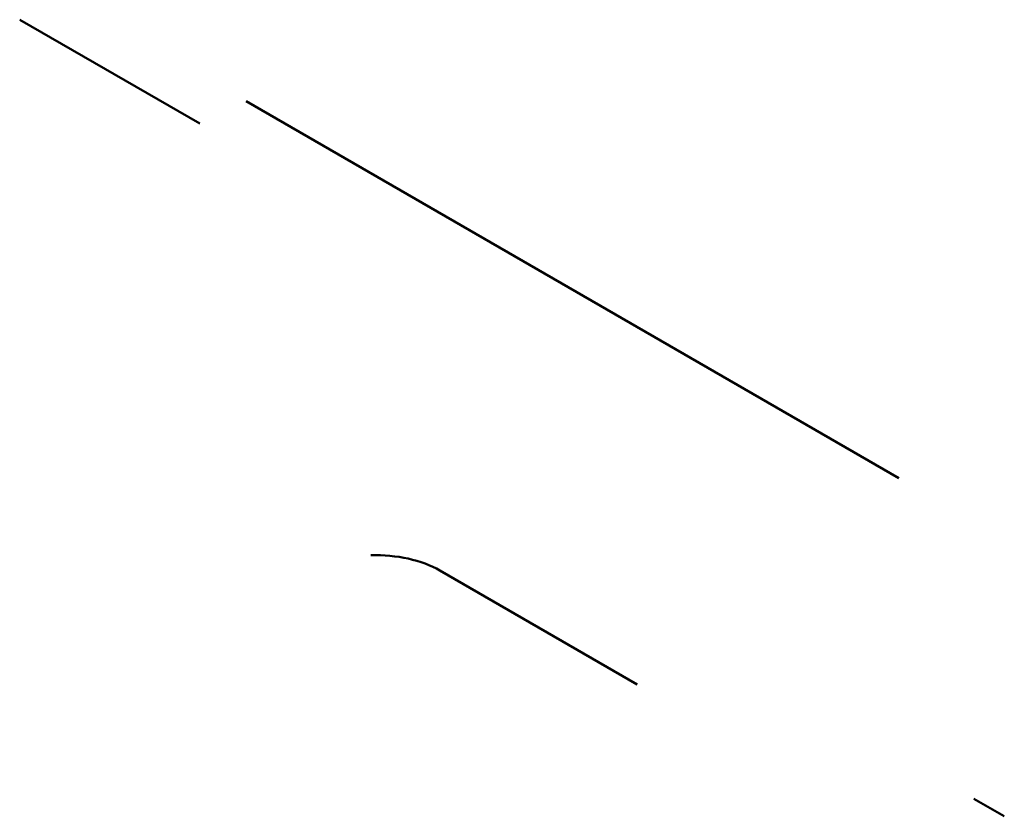
# Model space of a CAD drawing. Units: inches. Extents: x 666 to 20096, y 555 to 16161.
# Tile 2 of 2: x 18068 to 20096, y 14520 to 16161. Entities that reach past the tile are written whole.
import ezdxf

# ---------------------------------------------------------------- set-up
doc = ezdxf.new("R2010")
doc.units = ezdxf.units.IN
doc.header["$MEASUREMENT"] = 0
doc.layers.add('M-OUTL', color=7, linetype='Continuous', lineweight=50)

msp = doc.modelspace()

# ---------------------------------------------------------------- linework, layer by layer
at = {"layer": 'M-OUTL'}
for p, q in [((18438.6, 15947), (18067.8, 16161.1)), ((19879.4, 15216.8), (18534.4, 15993.3)), ((18933.5, 15026.3), (19339.9, 14791.7)), ((20096.4, 14520), (20033.6, 14556.2))]:
    msp.add_line(p, q, dxfattribs=at)
msp.add_ellipse((18801.6, 14950.1), major_axis=(186.7, 0), ratio=0.57735, start_param=0.785398, end_param=1.626467, dxfattribs=at)

doc.saveas('drawing.dxf')
